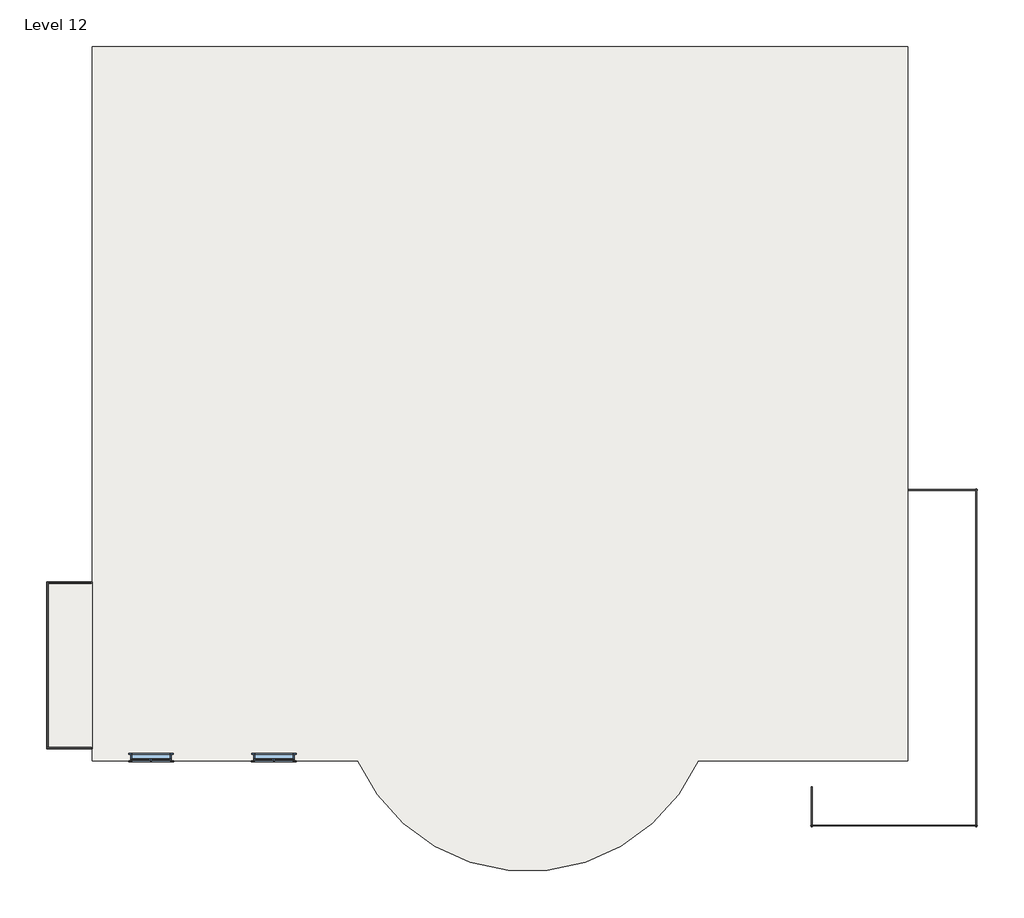
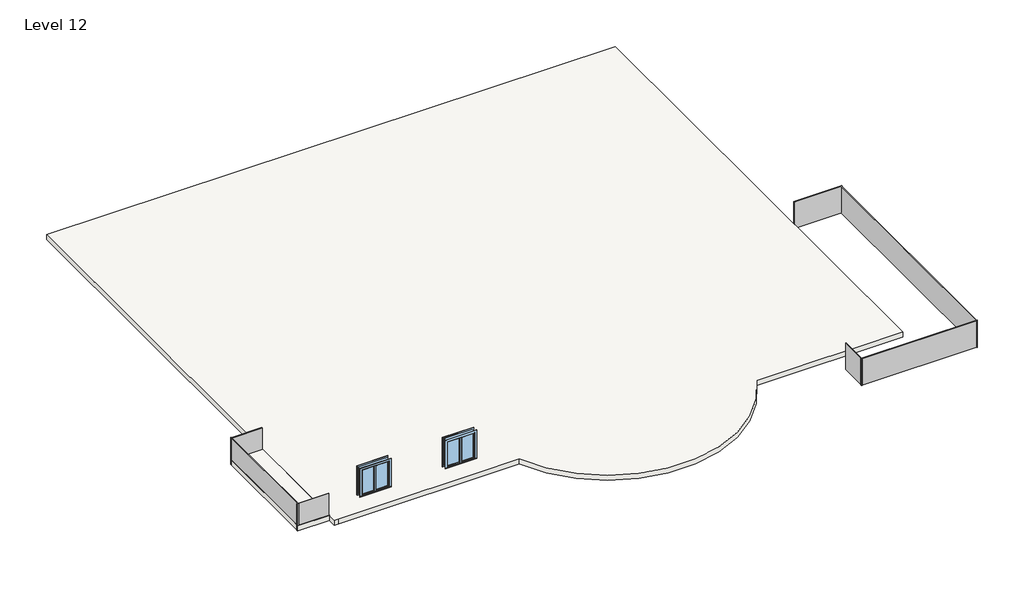
# One storey: 7 plates, 2 slabs, 2 windows.
"""IFC4 building model written with IfcOpenShell, lengths in millimetres."""

from ifc_helpers import new_model, si_unit, point, frame, frame_2d, origin, place, context, project, spatial, polyline, circle_curve, trimmed, segment, composite_curve, outline, extrude, transform, mapped, element, save
from components import system_panel_glazed_c55d8a5b, system_panel_glazed_a5f349e9, system_panel_glazed_61697952, system_panel_glazed_07392c36, system_panel_glazed_4fcd3a06, system_panel_glazed_fe6f5f94, system_panel_glazed_b1131520, window_0862ab64

model = new_model("IFC4")

# Units and contexts
model_context = context("Model", 3, world=origin())
ifc_project = project(units=[si_unit("LENGTHUNIT", "METRE", prefix="MILLI")], contexts=[model_context])

# Site, building, storey
site = spatial("IfcSite", under=ifc_project)
building = spatial("IfcBuilding", under=site)
storey = spatial("IfcBuildingStorey", under=building, Name="Level 12", Elevation=19431.0)

# Plates
placement = place(None, origin())
system_panel_glazed_shape = system_panel_glazed_c55d8a5b(model_context)
element("IfcPlate", 1, ObjectType="System Panel : Glazed", at=placement, inside=storey, context=model_context, shape_type="MappedRepresentation", body=[
    mapped(system_panel_glazed_shape, transform((7558.5964352, -16059.2808221, 19431.0), x_axis=(1.0, 0.0, 0.0), y_axis=(0.0, 1.0, 0.0), z_axis=(0.0, 0.0, 1.0))),
])
system_panel_glazed_2_shape = system_panel_glazed_a5f349e9(model_context)
element("IfcPlate", 2, ObjectType="System Panel : Glazed", at=placement, inside=storey, context=model_context, shape_type="MappedRepresentation", body=[
    mapped(system_panel_glazed_2_shape, transform((-17981.0459551, -11201.4489591, 19431.0), x_axis=(0.0, -1.0, 0.0), y_axis=(1.0, 0.0, 0.0), z_axis=(0.0, 0.0, 1.0))),
])
system_panel_glazed_3_shape = system_panel_glazed_61697952(model_context)
element("IfcPlate", 3, ObjectType="System Panel : Glazed", at=placement, inside=storey, context=model_context, shape_type="MappedRepresentation", body=[
    mapped(system_panel_glazed_3_shape, transform((-17307.1982489, -8690.0239591, 19431.0), x_axis=(-1.0, 0.0, 0.0), y_axis=(0.0, -1.0, 0.0), z_axis=(0.0, 0.0, 1.0))),
])
system_panel_glazed_4_shape = system_panel_glazed_07392c36(model_context)
element("IfcPlate", 4, ObjectType="System Panel : Glazed", at=placement, inside=storey, context=model_context, shape_type="MappedRepresentation", body=[
    mapped(system_panel_glazed_4_shape, transform((-17304.7709551, -13712.8739591, 19431.0), x_axis=(1.0, 0.0, 0.0), y_axis=(0.0, 1.0, 0.0), z_axis=(0.0, 0.0, 1.0))),
])
system_panel_glazed_5_shape = system_panel_glazed_4fcd3a06(model_context)
element("IfcPlate", 5, ObjectType="System Panel : Glazed", at=placement, inside=storey, context=model_context, shape_type="MappedRepresentation", body=[
    mapped(system_panel_glazed_5_shape, transform((9031.7964352, -5873.8808221, 19431.0), x_axis=(-1.0, 0.0, 0.0), y_axis=(0.0, -1.0, 0.0), z_axis=(0.0, 0.0, 1.0))),
])
system_panel_glazed_6_shape = system_panel_glazed_fe6f5f94(model_context)
element("IfcPlate", 6, ObjectType="System Panel : Glazed", at=placement, inside=storey, context=model_context, shape_type="MappedRepresentation", body=[
    mapped(system_panel_glazed_6_shape, transform((5043.9964352, -15458.7293258, 19431.0), x_axis=(0.0, -1.0, 0.0), y_axis=(1.0, 0.0, 0.0), z_axis=(0.0, 0.0, 1.0))),
])
system_panel_glazed_7_shape = system_panel_glazed_b1131520(model_context)
element("IfcPlate", 7, ObjectType="System Panel : Glazed", at=placement, inside=storey, context=model_context, shape_type="MappedRepresentation", body=[
    mapped(system_panel_glazed_7_shape, transform((10073.1964352, -10966.5808221, 19431.0), x_axis=(0.0, 1.0, 0.0), y_axis=(-1.0, 0.0, 0.0), z_axis=(0.0, 0.0, 1.0))),
])

# Slabs
element("IfcSlab", 8, ObjectType="9\"", at=placement, inside=storey, context=model_context, shape_type="SweptSolid", body=[
    extrude(outline(composite_curve([segment(polyline([(-16607.9505427, 7461.1191779), (7979.2494573, 7461.1191779), (7979.2494573, -14078.0808221), (1652.8739931, -14078.0808221)]), True, "CONTINUOUS"), segment(trimmed(circle_curve(frame_2d((-3476.1505427, -11788.3650223)), 5616.9111737), [point((1652.8739931, -14078.0808221))], [point((-8605.1750786, -14078.0808221))], False, "CARTESIAN"), True, "CONTINUOUS"), segment(polyline([(-8605.1750786, -14078.0808221), (-16404.7505427, -14078.0808221), (-16607.9505427, -14078.0808221), (-16607.9505427, 7461.1191779)]), True, "CONTINUOUS")], self_intersect=False)), frame((0.0, 0.0, 19431.0), z_axis=(0.0, 0.0, 1.0), x_axis=(1.0, 0.0, 0.0)), (0.0, 0.0, 1.0), 228.6),
])
element("IfcSlab", 9, ObjectType="9\"", at=placement, inside=storey, context=model_context, shape_type="SweptSolid", body=[
    extrude(outline(polyline([(-17972.8272291, -8690.0239591), (-16601.2272291, -8690.0239591), (-16601.2272291, -13719.2239591), (-17972.8272291, -13719.2239591), (-17972.8272291, -8690.0239591)])), frame((0.0, 0.0, 19431.0), z_axis=(0.0, 0.0, 1.0), x_axis=(1.0, 0.0, 0.0)), (0.0, 0.0, 1.0), 228.6),
])

# Windows
window_shape = window_0862ab64(model_context)
element("IfcWindow", 10, ObjectType="Casement Dbl with Trim : 48\" x 48\"", at=placement, inside=storey, context=model_context, shape_type="MappedRepresentation", body=[
    mapped(window_shape, transform((-14829.9505427, -13957.4308221, 19431.0), x_axis=(-1.0, 0.0, 0.0), y_axis=(0.0, -1.0, 0.0), z_axis=(0.0, 0.0, 1.0))),
])
element("IfcWindow", 11, ObjectType="Casement Dbl with Trim : 48\" x 48\"", at=placement, inside=storey, context=model_context, shape_type="MappedRepresentation", body=[
    mapped(window_shape, transform((-11129.6382271, -13957.4308221, 19431.0), x_axis=(-1.0, 0.0, 0.0), y_axis=(0.0, -1.0, 0.0), z_axis=(0.0, 0.0, 1.0))),
])

save(model, "model.ifc")

# Revit data of these elements
# Type "System Panel : Glazed"
#   Construction Type Id = "GSP4R"
#   Analytic Construction = "1/8 in Pilkington single glazing"
#   Visual Light Transmittance = 0.9
#   Solar Heat Gain Coefficient = 0.86
#   Heat Transfer Coefficient (U) = 1.18115 BTU/(h·ft²·°F)
# Type "9\""
#   Assembly Code = "B1010"
#   Function = 0
#   Layers, outside or top first: 0' - 9" no material (function 1)
# Type "Casement Dbl with Trim : 48\" x 48\""
#   Type Mark = "10"
#   Construction Type Id = "GSP4R"
#   Assembly Code = "B2020100"
#   Analytic Construction = "1/8 in Pilkington single glazing"
#   Visual Light Transmittance = 0.9
#   Solar Heat Gain Coefficient = 0.78
#   Heat Transfer Coefficient (U) = 0.6496 BTU/(h·ft²·°F)
#   Height = 4' - 0"
#   Default Sill Height = 3' - 0"
#   Trim Projection - Ext. = 0' - 0 1/2"
#   Trim Projection - Int. = 0' - 0 3/4"
#   Trim Width - Exterior = 0' - 3 1/2"
#   Trim Width - Interior = 0' - 3 1/2"
#   Width = 4' - 0"
#   Window Inset = 0' - 0 3/4"
#   Define Thermal Properties by = 1
#   Glass Pane Material = Glass
#   Sash Material = Sash
#   Trim Exterior Material = Trim
#   Trim Interior Material = Trim
#   Wall Closure = (empty or 0)
# Elements 1, 2, 3, 4, 5, 6, 7 (IfcPlate, "System Panel : Glazed")
#   Phase Created = New Construction
#   Materials on its faces: "Glass"
# Element 8 (IfcSlab, "9\"")
#   built-in parameter 1001955 = 1.5708 (stored number, unit not read)
#   Height Offset From Level = 0' - 9"
#   Phase Created = New Construction
#   Materials on its faces: "Default Floor"
# Element 9 (IfcSlab, "9\"")
#   built-in parameter 1001955 = 3.14159 (stored number, unit not read)
#   Height Offset From Level = 0' - 9"
#   Phase Created = New Construction
#   Materials on its faces: "Default Floor"
# Element 10 (IfcWindow, "Casement Dbl with Trim : 48\" x 48\"")
#   Mark = "35"
#   Phase Created = New Construction
#   Materials on its faces: "Sash", "Trim", "Glass"
# Element 11 (IfcWindow, "Casement Dbl with Trim : 48\" x 48\"")
#   Mark = "36"
#   Phase Created = New Construction
#   Materials on its faces: "Sash", "Trim", "Glass"
# Materials
#   "Glass": class "Glass", colour RGB 0 128 192, transparency 0.75, Description = "Soda Lime Glass", Cost = 0
#   "Sash": class "Wood", colour RGB 224 178 126, transparency 0
#   "Trim": class "Wood", colour RGB 224 178 126, transparency 0
#   "Default Floor": colour RGB 128 128 128, transparency 0
